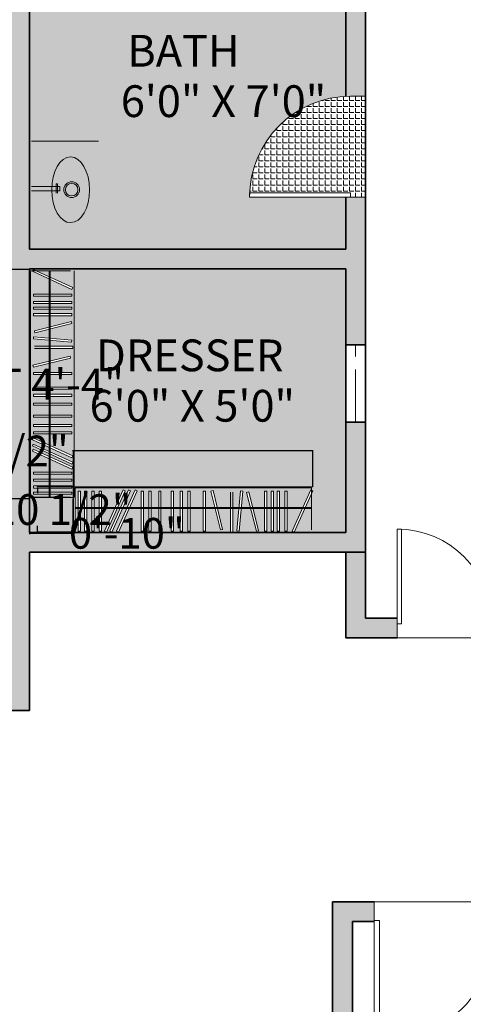
# Model space of a CAD drawing. Units: inches. Extents: x 2167 to 2589, y 1680 to 2489.
# Tile 36 of 38: x 2346 to 2447, y 2143 to 2367. Entities that reach past the tile are written whole.
import ezdxf

# ---------------------------------------------------------------- set-up
doc = ezdxf.new("R2010")
doc.units = ezdxf.units.IN
doc.header["$MEASUREMENT"] = 0
doc.linetypes.add('ACAD_ISO02W100', pattern=[15, 12, -3])
doc.layers.get('0').update_dxf_attribs({"color": 250})
for name, color, linetype, lineweight in [('A-ANNO-DIMS', 2, 'Continuous', 18), ('A-AREA-IDEN', 7, 'Continuous', 18), ('A-DOOR', 4, 'Continuous', 18), ('A-FLOR-FIXT', 8, 'Continuous', 18), ('A-FLOR-TILE-PATT', 252, 'Continuous', 13), ('A-WALL-OVHD', 8, 'ACAD_ISO02W100', 18), ('A-WALL-PATT', 250, 'Continuous', 13), ('closet', 250, 'Continuous', 18), ('walls', 7, 'Continuous', 35)]:
    doc.layers.add(name, color=color, linetype=linetype, lineweight=lineweight)
for name, color, linetype, lineweight, true_color in [('A-FLOR-FIXT-PATT', 7, 'Continuous', 13, 0xebebeb), ('A-FLOR-PATT', 254, 'Continuous', 13, 0xfeeab9), ('A-FURN-FIXD-PATT', 33, 'Continuous', 13, 0xcd8e5c)]:
    doc.layers.add(name, color=color, linetype=linetype, lineweight=lineweight, true_color=true_color)
doc.styles.get("Standard").update_dxf_attribs({"font": 'arial.ttf'})
doc.dimstyles.get("Standard").update_dxf_attribs({"dimtxt": 7, "dimasz": 0.18, "dimexe": 0.18, "dimexo": 0.0625, "dimgap": 0.09, "dimtad": 0, "dimtih": 1, "dimtoh": 1, "dimdec": 1, "dimzin": 0, "dimdsep": 46, "dimlunit": 3, "dimtxsty": 'Standard', "dimcen": 0.09, "dimadec": 0, "dimazin": 0, "dimtfac": 1, "dimtdec": 1, "dimtofl": 0, "dimtmove": 0, "dimatfit": 3, "dimfxl": 1, "dimtolj": 1, "dimtzin": 0, "dimarcsym": 0})
pattern_1 = [(0, (0, 0), (0, 1.375), [1, -0.375]), (90, (0, 0), (-1.375, 1e-16), [1, -0.375])]

# ---------------------------------------------------------------- blocks, each defined once
blk = doc.blocks.new('*U2')
for p, q in [((0, 0), (0, -6)), ((40, 0), (40, -6))]:
    blk.add_line(p, q)
blk.add_lwpolyline([(0, 0), (0, 40), (1.75, 40), (1.75, 0)], close=True)
blk.add_arc((0, 0), 40, 0, 90)
blk = doc.blocks.new('closet')
at = {"layer": 'closet'}
for p, q in [((-0.71, -5.58), (5.59, 8.19)), ((-0.23, 7.39), (-0.23, -6.57)), ((6.27, 7.88), (-0.04, -5.89)), ((5.59, 8.19), (6.27, 7.88)), ((7.92, 7.84), (8.68, 7.84)), ((7.92, 7.84), (7.92, -5.51)), ((8.68, 7.84), (8.68, -5.51)), ((10.44, 7.84), (11.2, 7.84)), ((10.44, 7.84), (10.44, -5.51)), ((11.2, 7.84), (11.2, -5.51)), ((12.45, 7.84), (13.21, 7.84)), ((12.45, 7.84), (12.45, -5.51)), ((13.21, 7.84), (13.21, -5.51)), ((14.71, 7.84), (15.47, 7.84)), ((14.71, 7.84), (14.71, -5.51)), ((15.47, 7.84), (15.47, -5.51)), ((17.44, 7.75), (18.17, 7.93)), ((17.44, 7.75), (20.73, -5.2)), ((18.17, 7.93), (21.46, -5.01)), ((23.92, 7.84), (22.75, -5.46)), ((24.67, 7.78), (23.51, -5.53)), ((23.92, 7.84), (24.67, 7.78)), ((26.09, 8.25), (26.09, -5.1)), ((26.84, 8.25), (26.84, -5.1)), ((29.49, 7.29), (32.64, -5.69)), ((30.22, 7.46), (33.37, -5.51)), ((35.23, 7.84), (35.23, -5.51)), ((35.99, 7.84), (35.99, -5.51)), ((40.33, 7.84), (40.33, -5.51)), ((41.08, 7.84), (41.08, -5.51)), ((42.85, 7.84), (42.85, -5.51)), ((43.61, 7.84), (43.61, -5.51)), ((45.9, 7.84), (45.9, -5.51)), ((46.65, 7.84), (46.65, -5.51)), ((50.07, 7.84), (50.07, -5.51)), ((50.82, 7.84), (50.82, -5.51)), ((53.32, 7.84), (53.32, -5.51)), ((54.08, 7.84), (54.08, -5.51)), ((55.9, 7.84), (55.9, -5.51)), ((56.65, 7.84), (56.65, -5.51)), ((57.99, -5.58), (64.3, 8.19)), ((64.97, 7.88), (58.67, -5.89)), ((60.19, -5.58), (66.49, 8.19)), ((67.17, 7.88), (60.87, -5.89)), ((62, -5.58), (68.3, 8.19)), ((68.98, 7.88), (62.67, -5.89)), ((69.96, 7.84), (69.96, -5.51)), ((70.72, 7.84), (70.72, -5.51)), ((72.43, 7.84), (72.43, -5.51)), ((73.19, 7.84), (73.19, -5.51)), ((74.82, 7.84), (74.82, -5.51)), ((75.57, 7.84), (75.57, -5.51)), ((76.94, 7.84), (76.94, -5.51)), ((77.69, 7.84), (77.69, -5.51)), ((56.23, 0.33), (0, 0.33)), ((56.2, 0), (0, 0)), ((56.2, 0), (78.76, 0)), ((56.23, 0.33), (78.76, 0.33)), ((-0.04, -5.89), (-0.71, -5.58)), ((21.46, -5.01), (20.73, -5.2)), ((23.51, -5.53), (22.75, -5.46)), ((33.37, -5.51), (32.64, -5.69)), ((35.99, -5.51), (35.23, -5.51)), ((41.08, -5.51), (40.33, -5.51)), ((43.61, -5.51), (42.85, -5.51)), ((46.65, -5.51), (45.9, -5.51)), ((50.82, -5.51), (50.07, -5.51)), ((54.08, -5.51), (53.32, -5.51)), ((56.65, -5.51), (55.9, -5.51)), ((58.67, -5.89), (57.99, -5.58)), ((60.87, -5.89), (60.19, -5.58)), ((62.67, -5.89), (62, -5.58)), ((70.72, -5.51), (69.96, -5.51)), ((73.19, -5.51), (72.43, -5.51)), ((75.57, -5.51), (74.82, -5.51)), ((77.69, -5.51), (76.94, -5.51))]:
    blk.add_line(p, q, dxfattribs=at)
blk = doc.blocks.new('rotated closet')
at = {"layer": 'closet'}
for p, q in [((26.32, 0.86), (27.07, 0.86)), ((29.72, -0.11), (30.45, 0.07)), ((35.46, 0.45), (36.22, 0.45)), ((40.56, 0.45), (41.31, 0.45)), ((43.08, 0.45), (43.84, 0.45)), ((46.13, 0.45), (46.88, 0.45)), ((50.3, 0.45), (51.05, 0.45)), ((53.56, 0.45), (54.31, 0.45)), ((56.13, 0.45), (56.88, 0.45)), ((64.53, 0.8), (65.2, 0.49)), ((66.72, 0.8), (67.4, 0.49)), ((68.53, 0.8), (69.21, 0.49)), ((70.19, 0.45), (70.95, 0.45)), ((72.66, 0.45), (73.42, 0.45)), ((75.05, 0.45), (75.81, 0.45)), ((77.17, 0.45), (77.92, 0.45)), ((78.99, 0), (78.99, -13.96)), ((8.91, -12.91), (8.15, -12.91)), ((11.43, -12.91), (10.67, -12.91)), ((13.44, -12.91), (12.68, -12.91)), ((15.7, -12.91), (14.94, -12.91)), ((-0.46, -14.27), (79.54, -14.27)), ((0, -13.96), (78.99, -13.96))]:
    blk.add_line(p, q, dxfattribs=at)
blk.add_blockref('closet', (0.23, -7.39), dxfattribs=at)
blk = doc.blocks.new('LAV-OVAL-WITH-TAP')
for p, q in [((6.14, 5.63), (6.14, 5.92)), ((6.14, 5.92), (8.26, 5.92)), ((8.26, 5.63), (6.14, 5.63)), ((7.69, 6.42), (6.74, 6.42)), ((6.74, 6.42), (6.74, 0)), ((7.69, 6.42), (7.69, 0))]:
    blk.add_line(p, q)
for radius in [1.79, 1.79, 1.43, 1.43, 1.43, 1.43]:
    blk.add_circle((7.46, 9.13), radius)
blk.add_ellipse((7.48, 8.9), major_axis=(7.48, 0.02), ratio=0.576535)
blk = doc.blocks.new('*D33')
at = {"layer": 'A-ANNO-DIMS', "color": 0, "lineweight": -2, "transparency": 16777216}
for p, q in [((2358.53, 2268.74), (2358.35, 2268.74)), ((2358.53, 2260.62), (2358.53, 2268.92)), ((2412.91, 2268.74), (2358.71, 2268.74)), ((2413.09, 2260.62), (2413.09, 2268.92))]:
    blk.add_line(p, q, dxfattribs=at)
at = {"layer": 'A-ANNO-DIMS', "color": 0, "transparency": 16777216}
for points in [[(2358.71, 2268.77), (2358.71, 2268.71), (2358.53, 2268.74)], [(2412.91, 2268.77), (2412.91, 2268.71), (2413.09, 2268.74)]]:
    blk.add_solid(points, dxfattribs=at)
at = {"layer": 'Defpoints', "color": 0, "transparency": 16777216}
for p in [(2358.53, 2268.74), (2358.53, 2260.56), (2413.09, 2260.56)]:
    blk.add_point(p, dxfattribs=at)
at = {"layer": 'A-ANNO-DIMS', "color": 0, "transparency": 16777216, "insert": (2319.92, 2268.74), "char_height": 7, "attachment_point": 5}
blk.add_mtext('\\A1;CLOSET 4\'-6 1/2"', dxfattribs=at)
blk = doc.blocks.new('*D34')
at = {"layer": 'A-ANNO-DIMS', "color": 0, "lineweight": -2, "transparency": 16777216}
for p, q in [((2358.47, 2260.56), (2350.17, 2260.56)), ((2350.35, 2260.38), (2350.35, 2259.11)), ((2350.35, 2250.42), (2350.35, 2251.69)), ((2358.47, 2250.24), (2350.17, 2250.24))]:
    blk.add_line(p, q, dxfattribs=at)
at = {"layer": 'A-ANNO-DIMS', "color": 0, "transparency": 16777216}
for points in [[(2350.32, 2260.38), (2350.38, 2260.38), (2350.35, 2260.56)], [(2350.32, 2250.42), (2350.38, 2250.42), (2350.35, 2250.24)]]:
    blk.add_solid(points, dxfattribs=at)
at = {"layer": 'Defpoints', "color": 0, "transparency": 16777216}
for p in [(2358.53, 2260.56), (2350.35, 2250.24), (2358.53, 2250.24)]:
    blk.add_point(p, dxfattribs=at)
at = {"layer": 'A-ANNO-DIMS', "color": 0, "transparency": 16777216, "insert": (2350.35, 2255.4), "char_height": 7, "attachment_point": 5}
blk.add_mtext('\\A1;0\'-10 1/2"', dxfattribs=at)
blk = doc.blocks.new('*D37')
at = {"layer": 'A-ANNO-DIMS', "color": 0, "lineweight": -2, "transparency": 16777216}
for p, q in [((2348.49, 2310.05), (2340.54, 2310.05)), ((2340.72, 2309.87), (2340.72, 2287.66)), ((2340.72, 2258.02), (2340.72, 2280.23)), ((2348.49, 2257.84), (2340.54, 2257.84))]:
    blk.add_line(p, q, dxfattribs=at)
at = {"layer": 'A-ANNO-DIMS', "color": 0, "transparency": 16777216}
for points in [[(2340.69, 2309.87), (2340.75, 2309.87), (2340.72, 2310.05)], [(2340.69, 2258.02), (2340.75, 2258.02), (2340.72, 2257.84)]]:
    blk.add_solid(points, dxfattribs=at)
at = {"layer": 'Defpoints', "color": 0, "transparency": 16777216}
for p in [(2348.55, 2310.05), (2340.72, 2257.84), (2348.55, 2257.84)]:
    blk.add_point(p, dxfattribs=at)
at = {"layer": 'A-ANNO-DIMS', "color": 0, "transparency": 16777216, "insert": (2340.72, 2283.95), "char_height": 7, "attachment_point": 5}
blk.add_mtext('\\A1;CLOSET 4\'-4"', dxfattribs=at)
blk = doc.blocks.new('*D38')
at = {"layer": 'A-ANNO-DIMS', "color": 0, "lineweight": -2, "transparency": 16777216}
for p, q in [((2348.55, 2257.78), (2348.55, 2249.83)), ((2358.42, 2257.78), (2358.42, 2249.83)), ((2348.73, 2250.01), (2358.24, 2250.01)), ((2358.42, 2250.01), (2358.6, 2250.01))]:
    blk.add_line(p, q, dxfattribs=at)
at = {"layer": 'A-ANNO-DIMS', "color": 0, "transparency": 16777216}
for points in [[(2348.73, 2250.04), (2348.73, 2249.98), (2348.55, 2250.01)], [(2358.24, 2250.04), (2358.24, 2249.98), (2358.42, 2250.01)]]:
    blk.add_solid(points, dxfattribs=at)
at = {"layer": 'Defpoints', "color": 0, "transparency": 16777216}
for p in [(2348.55, 2257.84), (2358.42, 2257.84), (2358.42, 2250.01)]:
    blk.add_point(p, dxfattribs=at)
at = {"layer": 'A-ANNO-DIMS', "color": 0, "transparency": 16777216, "insert": (2370.71, 2250.01), "char_height": 7, "attachment_point": 5}
blk.add_mtext('\\A1;0\'-10"', dxfattribs=at)

msp = doc.modelspace()

# ---------------------------------------------------------------- hatches: boundary and pattern name
at = {"layer": 'A-FLOR-FIXT-PATT'}
h = msp.add_hatch(color=256, dxfattribs=at)
h.dxf.hatch_style = 1
edge = h.paths.add_edge_path()
edge.add_line((2364.26, 2318.3), (2364.26, 2339.2))
edge.add_line((2364.26, 2339.2), (2349, 2339.2))
edge.add_line((2349, 2339.2), (2349, 2328.91))
edge.add_line((2349, 2328.91), (2353.6, 2328.91))
edge.add_ellipse((2357.9, 2328.17), major_axis=(0.02, -7.48), ratio=0.576535, start_angle=272.6137, end_angle=620.1108, ccw=False)
edge.add_line((2353.59, 2327.96), (2349, 2327.96))
edge.add_line((2349, 2327.96), (2349, 2318.3))
edge.add_line((2349, 2318.3), (2364.26, 2318.3))
h = msp.add_hatch(color=256, dxfattribs=at)
h.dxf.hatch_style = 1
edge = h.paths.add_edge_path()
edge.add_ellipse((2357.9, 2328.17), major_axis=(0.02, -7.48), ratio=0.576535, start_angle=272.6137, end_angle=260.1108)
edge.add_line((2353.6, 2328.91), (2354.63, 2328.91))
edge.add_line((2354.63, 2328.91), (2354.63, 2329.51))
edge.add_line((2354.63, 2329.51), (2354.92, 2329.51))
edge.add_line((2354.92, 2329.51), (2354.92, 2328.91))
edge.add_line((2354.92, 2328.91), (2355.42, 2328.91))
edge.add_line((2355.42, 2328.91), (2355.42, 2327.96))
edge.add_line((2355.42, 2327.96), (2353.59, 2327.96))
h.paths.add_polyline_path([(2358.14, 2326.4, -1), (2358.14, 2329.97, -1)], flags=16)
h.paths.add_polyline_path([(2358.14, 2329.61, -1), (2358.14, 2326.76, -1)], flags=0)
h.paths.add_polyline_path([(2358.14, 2326.76, 1), (2358.14, 2329.61, 1)], flags=0)
edge = h.paths.add_edge_path()
edge.add_line((2354.63, 2327.96), (2354.63, 2328.91))
edge.add_line((2354.63, 2328.91), (2353.6, 2328.91))
edge.add_ellipse((2357.9, 2328.17), major_axis=(0.02, -7.48), ratio=0.576535, start_angle=260.1108, end_angle=272.6137)
edge.add_line((2353.59, 2327.96), (2354.63, 2327.96))
h.paths.add_polyline_path([(2355.42, 2327.96), (2355.42, 2328.91), (2354.92, 2328.91), (2354.92, 2327.96)], flags=17)
h.paths.add_polyline_path([(2354.92, 2327.96), (2354.92, 2328.91), (2354.63, 2328.91), (2354.63, 2327.96)], flags=17)
h.paths.add_polyline_path([(2354.92, 2328.91), (2354.92, 2329.51), (2354.63, 2329.51), (2354.63, 2328.91)], flags=17)
edge = h.paths.add_edge_path()
edge.add_ellipse((2357.9, 2328.17), major_axis=(0.02, -7.48), ratio=0.576535, start_angle=260.1108, end_angle=272.6137, ccw=False)
edge.add_line((2353.6, 2328.91), (2349, 2328.91))
edge.add_line((2349, 2328.91), (2349, 2327.96))
edge.add_line((2349, 2327.96), (2353.59, 2327.96))
h = msp.add_hatch(color=256, dxfattribs=at)
h.dxf.hatch_style = 1
h.paths.add_polyline_path([(2358.14, 2329.61, 1), (2358.14, 2326.76, 1)], flags=0)
h.paths.add_polyline_path([(2358.14, 2329.97, 1), (2358.14, 2326.4, 1)])
h.paths.add_polyline_path([(2358.14, 2329.61, -1), (2358.14, 2326.76, -1)], flags=16)
h = msp.add_hatch(color=256, dxfattribs=at)
h.dxf.hatch_style = 1
h.paths.add_polyline_path([(2358.14, 2329.61, 1), (2358.14, 2326.76, 1)])
at = {"layer": 'A-FLOR-PATT'}
h = msp.add_hatch(color=256, dxfattribs=at)
h.dxf.hatch_style = 1
h.paths.add_polyline_path([(2420.55, 2310.19), (2349.46, 2310.19), (2349.4, 2310.05), (2350.08, 2309.74), (2353.25, 2309.74), (2353.25, 2308.29), (2358.7, 2305.79), (2358.7, 2260.56), (2412.76, 2260.56), (2412.76, 2259.82), (2413.09, 2259.67), (2412.76, 2258.96), (2412.76, 2255.64), (2411.24, 2255.64), (2408.75, 2250.19), (2420.55, 2250.19)])
at = {"layer": 'A-FLOR-TILE-PATT'}
h = msp.add_hatch(dxfattribs=at)
h.set_pattern_fill('ANGLE', color=256, scale=5)
h.set_pattern_definition(pattern_1)
h.paths.add_polyline_path([(2420.55, 2398.69), (2348.55, 2398.69), (2348.55, 2314.69), (2420.55, 2314.69), (2420.55, 2326.49), (2398.64, 2326.49), (2398.64, 2327.5), (2398.66, 2327.5, -0.388161), (2420.55, 2349.43)])
h.paths.add_polyline_path([(2379.26, 2371.69), (2358.26, 2371.69), (2358.26, 2373.69), (2358.76, 2373.69), (2358.76, 2383.69), (2358.26, 2383.69), (2358.26, 2385.69), (2358.76, 2385.69, -0.206081), (2365.76, 2391.29), (2365.76, 2393.69), (2364.76, 2393.69), (2364.76, 2394.69), (2362.76, 2394.69), (2362.76, 2395.69), (2374.76, 2395.69), (2374.76, 2394.69), (2372.76, 2394.69), (2372.76, 2393.69), (2371.76, 2393.69), (2371.76, 2391.29, -0.206081), (2378.76, 2385.69), (2379.26, 2385.69), (2379.26, 2383.69), (2378.76, 2383.69), (2378.76, 2373.69), (2379.26, 2373.69)], flags=16)
edge = h.paths.add_edge_path(flags=16)
edge.add_ellipse((2357.9, 2328.17), major_axis=(0.02, -7.48), ratio=0.576535, start_angle=272.6137, end_angle=620.1108, ccw=False)
edge.add_ellipse((2357.9, 2328.17), major_axis=(0.02, -7.48), ratio=0.576535, start_angle=260.1108, end_angle=272.6137, ccw=False)
h.paths.add_polyline_path([(2359.92, 2328.19, -1), (2356.35, 2328.19, -1)], flags=0)
h.paths.add_polyline_path([(2356.71, 2328.19, -1), (2359.56, 2328.19, -1)], flags=0)
h.paths.add_polyline_path([(2355.42, 2328.91), (2355.42, 2327.96), (2354.63, 2327.96), (2354.63, 2329.51), (2354.92, 2329.51), (2354.92, 2328.91)], flags=0)
h = msp.add_hatch(dxfattribs=at)
h.set_pattern_fill('ANGLE', color=256, scale=5)
h.set_pattern_definition(pattern_1)
h.paths.add_polyline_path([(2425.05, 2349.45), (2421.6, 2349.45, 0.401453), (2398.66, 2327.5), (2421.6, 2327.5), (2421.6, 2326.49), (2425.05, 2326.49)])
at = {"layer": 'A-FURN-FIXD-PATT'}
h = msp.add_hatch(color=256, dxfattribs=at)
h.dxf.hatch_style = 1
h.paths.add_polyline_path([(2349.2, 2268.7), (2349.4, 2269.14), (2353.04, 2267.47), (2353.04, 2268.12), (2349.2, 2269.88), (2349.4, 2270.32), (2353.04, 2268.65), (2353.04, 2269.55), (2349.2, 2271.31), (2349.4, 2271.75), (2353.04, 2270.08), (2353.04, 2272.63), (2349.44, 2272.63), (2349.44, 2273.12), (2353.04, 2273.12), (2353.04, 2274.3), (2349.44, 2274.3), (2349.44, 2274.8), (2353.04, 2274.8), (2353.04, 2276.43), (2349.44, 2276.43), (2349.44, 2276.92), (2353.04, 2276.92), (2353.04, 2279.15), (2349.44, 2279.15), (2349.44, 2279.64), (2353.04, 2279.64), (2353.04, 2281.14), (2349.44, 2281.14), (2349.44, 2281.63), (2353.04, 2281.63), (2353.04, 2282.78), (2349.44, 2282.78), (2349.44, 2283.28), (2353.04, 2283.28), (2353.04, 2286.11), (2349.44, 2286.11), (2349.44, 2286.6), (2353.04, 2286.6), (2353.04, 2288.69), (2349.44, 2287.81), (2349.32, 2288.29), (2353.04, 2289.2), (2353.04, 2293.93), (2349.43, 2294.25), (2349.47, 2294.74), (2353.04, 2294.43), (2353.04, 2296.42), (2349.77, 2295.58), (2349.65, 2296.06), (2353.04, 2296.93), (2353.04, 2299.5), (2349.44, 2299.5), (2349.44, 2299.99), (2353.04, 2299.99), (2353.04, 2300.97), (2349.44, 2300.97), (2349.44, 2301.47), (2353.04, 2301.47), (2353.04, 2302.28), (2349.44, 2302.28), (2349.44, 2302.77), (2353.04, 2302.77), (2353.04, 2303.93), (2349.44, 2303.93), (2349.44, 2304.42), (2353.04, 2304.42), (2353.04, 2307.85), (2349.2, 2309.61), (2349.25, 2309.74), (2348.75, 2309.74), (2348.75, 2258.2), (2353.04, 2258.2), (2353.04, 2258.9), (2349.44, 2258.9), (2349.44, 2259.39), (2353.04, 2259.39), (2353.04, 2260.28), (2349.44, 2260.28), (2349.44, 2260.77), (2353.04, 2260.77), (2353.04, 2261.84), (2349.44, 2261.84), (2349.44, 2262.33), (2353.04, 2262.33), (2353.04, 2263.45), (2349.44, 2263.45), (2349.44, 2263.94), (2353.04, 2263.94), (2353.04, 2266.94)])
h.paths.add_polyline_path([(2353.25, 2266.84), (2353.25, 2263.94), (2358.15, 2263.94), (2358.15, 2263.45), (2353.25, 2263.45), (2353.25, 2262.33), (2358.15, 2262.33), (2358.15, 2261.84), (2353.25, 2261.84), (2353.25, 2260.77), (2358.15, 2260.77), (2358.15, 2260.28), (2353.25, 2260.28), (2353.25, 2259.39), (2358.15, 2259.39), (2358.15, 2258.9), (2353.25, 2258.9), (2353.25, 2258.2), (2357.86, 2258.2), (2358.42, 2258.2), (2358.7, 2258.2), (2358.7, 2309.74), (2350.08, 2309.74), (2358.38, 2305.94), (2358.18, 2305.5), (2353.25, 2307.75), (2353.25, 2304.42), (2358.15, 2304.42), (2358.15, 2303.93), (2353.25, 2303.93), (2353.25, 2302.77), (2358.15, 2302.77), (2358.15, 2302.28), (2353.25, 2302.28), (2353.25, 2301.47), (2358.15, 2301.47), (2358.15, 2300.97), (2353.25, 2300.97), (2353.25, 2299.99), (2358.15, 2299.99), (2358.15, 2299.5), (2353.25, 2299.5), (2353.25, 2296.98), (2358.09, 2298.21), (2358.21, 2297.73), (2353.25, 2296.47), (2353.25, 2294.41), (2358.15, 2293.98), (2358.11, 2293.49), (2353.25, 2293.91), (2353.25, 2292.57), (2358.42, 2292.57), (2358.42, 2292.07), (2353.25, 2292.07), (2353.25, 2289.25), (2357.79, 2290.35), (2357.91, 2289.87), (2353.25, 2288.74), (2353.25, 2286.6), (2358.15, 2286.6), (2358.15, 2286.11), (2353.25, 2286.11), (2353.25, 2283.28), (2358.15, 2283.28), (2358.15, 2282.78), (2353.25, 2282.78), (2353.25, 2281.63), (2358.15, 2281.63), (2358.15, 2281.14), (2353.25, 2281.14), (2353.25, 2279.64), (2358.15, 2279.64), (2358.15, 2279.15), (2353.25, 2279.15), (2353.25, 2276.92), (2358.15, 2276.92), (2358.15, 2276.43), (2353.25, 2276.43), (2353.25, 2274.8), (2358.15, 2274.8), (2358.15, 2274.3), (2353.25, 2274.3), (2353.25, 2273.12), (2358.15, 2273.12), (2358.15, 2272.63), (2353.25, 2272.63), (2353.25, 2269.98), (2358.38, 2267.64), (2358.18, 2267.2), (2353.25, 2269.45), (2353.25, 2268.55), (2358.38, 2266.21), (2358.18, 2265.76), (2353.25, 2268.02), (2353.25, 2267.37), (2358.38, 2265.02), (2358.18, 2264.58)])
h = msp.add_hatch(color=256, dxfattribs=at)
h.dxf.hatch_style = 1
h.paths.add_polyline_path([(2369.87, 2259.88), (2370.33, 2259.67), (2368.59, 2255.87), (2369.27, 2255.87), (2371.11, 2259.88), (2371.57, 2259.67), (2369.83, 2255.87), (2370.77, 2255.87), (2372.6, 2259.88), (2373.06, 2259.67), (2371.32, 2255.87), (2373.98, 2255.87), (2373.98, 2259.63), (2374.49, 2259.63), (2374.49, 2255.87), (2375.73, 2255.87), (2375.73, 2259.63), (2376.25, 2259.63), (2376.25, 2255.87), (2377.95, 2255.87), (2377.95, 2259.63), (2378.47, 2259.63), (2378.47, 2255.87), (2380.8, 2255.87), (2380.8, 2259.63), (2381.31, 2259.63), (2381.31, 2255.87), (2382.87, 2255.87), (2382.87, 2259.63), (2383.39, 2259.63), (2383.39, 2255.87), (2384.59, 2255.87), (2384.59, 2259.63), (2385.11, 2259.63), (2385.11, 2255.87), (2388.07, 2255.87), (2388.07, 2259.63), (2388.58, 2259.63), (2388.58, 2255.87), (2390.76, 2255.87), (2389.85, 2259.63), (2390.35, 2259.75), (2391.29, 2255.87), (2396.25, 2255.87), (2396.57, 2259.64), (2397.09, 2259.59), (2396.76, 2255.87), (2398.84, 2255.87), (2397.97, 2259.28), (2398.47, 2259.41), (2399.37, 2255.87), (2402.06, 2255.87), (2402.06, 2259.63), (2402.57, 2259.63), (2402.57, 2255.87), (2403.6, 2255.87), (2403.6, 2259.63), (2404.11, 2259.63), (2404.11, 2255.87), (2404.97, 2255.87), (2404.97, 2259.63), (2405.48, 2259.63), (2405.48, 2255.87), (2406.69, 2255.87), (2406.69, 2259.63), (2407.2, 2259.63), (2407.2, 2255.87), (2410.79, 2255.87), (2412.63, 2259.88), (2412.76, 2259.82), (2412.76, 2260.35), (2358.91, 2260.35), (2358.91, 2255.87), (2359.63, 2255.87), (2359.63, 2259.63), (2360.15, 2259.63), (2360.15, 2255.87), (2361.08, 2255.87), (2361.08, 2259.63), (2361.6, 2259.63), (2361.6, 2255.87), (2362.71, 2255.87), (2362.71, 2259.63), (2363.22, 2259.63), (2363.22, 2255.87), (2364.39, 2255.87), (2364.39, 2259.63), (2364.9, 2259.63), (2364.9, 2255.87), (2368.04, 2255.87)])
h.paths.add_polyline_path([(2367.93, 2255.64), (2364.9, 2255.64), (2364.9, 2250.52), (2364.39, 2250.52), (2364.39, 2255.64), (2363.22, 2255.64), (2363.22, 2250.52), (2362.71, 2250.52), (2362.71, 2255.64), (2361.6, 2255.64), (2361.6, 2250.52), (2361.08, 2250.52), (2361.08, 2255.64), (2360.15, 2255.64), (2360.15, 2250.52), (2359.63, 2250.52), (2359.63, 2255.64), (2358.91, 2255.64), (2358.91, 2250.83), (2358.91, 2250.25), (2358.91, 2249.95), (2412.76, 2249.95), (2412.76, 2258.96), (2408.79, 2250.28), (2408.33, 2250.5), (2410.68, 2255.64), (2407.2, 2255.64), (2407.2, 2250.52), (2406.69, 2250.52), (2406.69, 2255.64), (2405.48, 2255.64), (2405.48, 2250.52), (2404.97, 2250.52), (2404.97, 2255.64), (2404.11, 2255.64), (2404.11, 2250.52), (2403.6, 2250.52), (2403.6, 2255.64), (2402.57, 2255.64), (2402.57, 2250.52), (2402.06, 2250.52), (2402.06, 2255.64), (2399.43, 2255.64), (2400.71, 2250.59), (2400.21, 2250.46), (2398.9, 2255.64), (2396.74, 2255.64), (2396.3, 2250.52), (2395.78, 2250.57), (2396.23, 2255.64), (2394.82, 2255.64), (2394.82, 2250.24), (2394.3, 2250.24), (2394.3, 2255.64), (2391.35, 2255.64), (2392.5, 2250.9), (2392, 2250.78), (2390.82, 2255.64), (2388.58, 2255.64), (2388.58, 2250.52), (2388.07, 2250.52), (2388.07, 2255.64), (2385.11, 2255.64), (2385.11, 2250.52), (2384.59, 2250.52), (2384.59, 2255.64), (2383.39, 2255.64), (2383.39, 2250.52), (2382.87, 2250.52), (2382.87, 2255.64), (2381.31, 2255.64), (2381.31, 2250.52), (2380.8, 2250.52), (2380.8, 2255.64), (2378.47, 2255.64), (2378.47, 2250.52), (2377.95, 2250.52), (2377.95, 2255.64), (2376.25, 2255.64), (2376.25, 2250.52), (2375.73, 2250.52), (2375.73, 2255.64), (2374.49, 2255.64), (2374.49, 2250.52), (2373.98, 2250.52), (2373.98, 2255.64), (2371.22, 2255.64), (2368.77, 2250.28), (2368.31, 2250.5), (2370.66, 2255.64), (2369.72, 2255.64), (2367.27, 2250.28), (2366.81, 2250.5), (2369.17, 2255.64), (2368.49, 2255.64), (2366.04, 2250.28), (2365.58, 2250.5)])
h = msp.add_hatch(color=256, dxfattribs=at)
h.dxf.hatch_style = 1
h.paths.add_polyline_path([(2358.48, 2258.16), (2348.55, 2258.16), (2348.55, 2257.84), (2348.55, 2250.19), (2358.48, 2250.19)])
at = {"layer": 'A-WALL-PATT'}
h = msp.add_hatch(color=256, dxfattribs=at)
h.dxf.hatch_style = 1
h.paths.add_polyline_path([(2471.54, 2407.69), (2405.59, 2407.69), (2405.59, 2398.69), (2420.55, 2398.69), (2420.55, 2349.43, -0.011499), (2421.6, 2349.45), (2425.05, 2349.45), (2425.05, 2398.69), (2471.54, 2398.69)])
h.paths.add_polyline_path([(2420.55, 2250.19), (2348.55, 2250.19), (2348.55, 2310.19), (2420.55, 2310.19)], flags=16)
h.paths.add_polyline_path([(2320.06, 2212.92, -0.014764), (2320.1, 2214.19), (2224.05, 2214.19), (2224.05, 2346.19), (2250.86, 2346.19), (2250.86, 2350.69), (2224.05, 2350.69), (2224.05, 2398.69), (2250.76, 2398.69), (2250.76, 2407.69), (2215.05, 2407.69), (2215.05, 2179.66), (2218.49, 2179.66), (2224.05, 2179.66), (2224.05, 2209.69), (2314.05, 2209.69), (2314.05, 2202.4), (2314.78, 2202.4), (2318.55, 2202.4), (2318.55, 2209.69), (2320.06, 2209.69)])
h.paths.add_polyline_path([(2310.92, 2349.42, -0.014764), (2310.96, 2350.69), (2297.23, 2350.69), (2297.23, 2346.19), (2310.92, 2346.19)], flags=17)
h.paths.add_polyline_path([(2425.05, 2275.27), (2420.55, 2275.27), (2420.55, 2292.87), (2425.05, 2292.87), (2425.05, 2326.49), (2421.6, 2326.49), (2420.55, 2326.49), (2420.55, 2314.69), (2348.55, 2314.69), (2348.55, 2398.69), (2373.55, 2398.69), (2373.55, 2404.36), (2373.55, 2407.69), (2297.68, 2407.69), (2297.68, 2398.69), (2344.05, 2398.69), (2344.05, 2350.69), (2332.45, 2350.69), (2332.45, 2349.42), (2332.45, 2346.19), (2344.05, 2346.19), (2344.05, 2214.19), (2341.59, 2214.19), (2341.59, 2212.92), (2341.59, 2209.69), (2348.55, 2209.69), (2348.55, 2245.69), (2425.05, 2245.69)])
h = msp.add_hatch(color=256, dxfattribs=at)
h.dxf.hatch_style = 1
h.paths.add_polyline_path([(2575.05, 2029.69), (2422.05, 2029.69), (2422.05, 2161.69), (2427.02, 2161.69), (2427.02, 2161.94), (2427.02, 2166.19), (2417.55, 2166.19), (2417.55, 2025.19), (2575.05, 2025.19)])
h.paths.add_polyline_path([(2575.05, 2166.19), (2503.01, 2166.19), (2503.01, 2161.69), (2575.05, 2161.69)], flags=17)
h.paths.add_polyline_path([(2575.05, 2161.69), (2566.05, 2161.69), (2566.05, 2029.69), (2575.05, 2029.69)], flags=17)
h.paths.add_polyline_path([(2575.05, 2025.19), (2566.05, 2025.19), (2566.05, 1869.19), (2575.05, 1869.19)])
h.paths.add_polyline_path([(2575.05, 1869.19), (2566.05, 1869.19), (2447.7, 1869.19, -0.014764), (2447.74, 1867.92), (2447.74, 1864.69), (2575.05, 1864.69)])
h.paths.add_polyline_path([(2530.05, 1864.69), (2525.55, 1864.69), (2525.55, 1816.69), (2452.05, 1816.69), (2452.05, 1812.19), (2530.05, 1812.19)])
h.paths.add_polyline_path([(2455.04, 1830.65), (2452.05, 1830.65), (2452.05, 1816.69), (2455.04, 1816.69)], flags=17)
h.paths.add_polyline_path([(2575.05, 1864.69), (2566.05, 1864.69), (2566.05, 1788.19), (2456.1, 1788.19), (2456.1, 1783.94, -0.042065), (2455.7, 1779.19), (2527.68, 1779.19), (2527.68, 1687.69), (2532.18, 1687.69), (2532.18, 1779.19), (2575.05, 1779.19)])
h.paths.add_polyline_path([(2421.87, 1696.69), (2416.11, 1696.69), (2416.11, 1687.69), (2421.87, 1687.69)])
h.paths.add_polyline_path([(2375.61, 1696.69), (2369.84, 1696.69), (2369.84, 1687.69), (2375.61, 1687.69)])
h.paths.add_polyline_path([(2425.05, 2245.69), (2420.55, 2245.69), (2420.55, 2226.19), (2432.29, 2226.19), (2432.29, 2229.42), (2432.29, 2230.69), (2425.05, 2230.69)])
h.paths.add_polyline_path([(2224.05, 2151.19), (2318.55, 2151.19), (2318.55, 2177.3), (2314.78, 2177.3, -0.007324), (2314.05, 2177.32), (2314.05, 2155.69), (2224.05, 2155.69), (2224.05, 2157.46), (2215.05, 2157.46), (2215.05, 2103.59), (2218.97, 2103.59), (2224.05, 2103.59)])

# ---------------------------------------------------------------- linework, layer by layer
at = {"layer": 'A-DOOR'}
for p, q in [((2432.29, 2226.19), (2453.82, 2226.19)), ((2427.02, 2166.19), (2455.38, 2166.19))]:
    msp.add_line(p, q, dxfattribs=at)
at = {"layer": 'A-FLOR-FIXT'}
msp.add_line((2364.26, 2339.2), (2349, 2339.2), dxfattribs=at)
at = {"layer": 'A-WALL-OVHD'}
msp.add_line((2422.8, 2275.27), (2422.8, 2292.87), dxfattribs=at)
at = {"layer": 'closet'}
for p, q in [((2348.55, 2257.84), (2348.55, 2310.04)), ((2348.75, 2309.74), (2348.75, 2258.2)), ((2348.75, 2309.74), (2357.86, 2309.74)), ((2358.7, 2309.74), (2358.7, 2258.16)), ((2358.48, 2260.77), (2358.15, 2260.77)), ((2358.48, 2250.19), (2358.48, 2260.77)), ((2358.53, 2260.56), (2413.07, 2260.56)), ((2358.53, 2260.56), (2358.53, 2250.19)), ((2358.7, 2258.16), (2358.7, 2260.56)), ((2412.76, 2260.35), (2358.91, 2260.35)), ((2412.76, 2260.35), (2412.76, 2250.83)), ((2358.47, 2258.16), (2348.55, 2258.16)), ((2348.55, 2258.16), (2348.55, 2257.84)), ((2348.75, 2258.2), (2357.86, 2258.2))]:
    msp.add_line(p, q, dxfattribs=at)
at = {"layer": 'walls'}
for p, q in [((2348.55, 2314.69), (2348.55, 2398.69)), ((2420.55, 2349.43), (2420.55, 2398.69)), ((2425.05, 2230.69), (2425.05, 2398.69)), ((2420.55, 2314.69), (2420.55, 2326.49)), ((2348.55, 2314.69), (2420.55, 2314.69)), ((2348.55, 2310.19), (2420.55, 2310.19)), ((2348.55, 2250.19), (2348.55, 2310.19)), ((2420.55, 2250.19), (2420.55, 2310.19)), ((2420.55, 2292.87), (2425.05, 2292.87)), ((2420.55, 2275.27), (2425.05, 2275.27)), ((2348.55, 2250.19), (2420.55, 2250.19)), ((2348.55, 2209.69), (2348.55, 2245.69)), ((2348.55, 2245.69), (2425.05, 2245.69)), ((2420.55, 2226.19), (2420.55, 2245.69)), ((2425.05, 2230.69), (2432.29, 2230.69)), ((2420.55, 2226.19), (2432.29, 2226.19)), ((2318.55, 2209.69), (2348.55, 2209.69)), ((2417.55, 2166.19), (2427.02, 2166.19)), ((2417.55, 2166.19), (2417.55, 2025.19)), ((2422.05, 2161.69), (2427.02, 2161.69)), ((2422.05, 2161.69), (2422.05, 2029.69))]:
    msp.add_line(p, q, dxfattribs=at)

# ---------------------------------------------------------------- block references
at = {"layer": 'A-DOOR'}
for p, xscale, yscale, zscale, rotation in [((2421.6, 2326.49), 0.5740396890227921, 0.5740396890227921, 0.5740396890227921, 90), ((2427.02, 2161.94), -0.7089553820317277, 0.7089553820317277, 0.7089553820317277, 180)]:
    msp.add_blockref('*U2', p, dxfattribs=dict(at, xscale=xscale, yscale=yscale, zscale=zscale, rotation=rotation))
at = {"layer": 'A-DOOR', "xscale": 0.5382298898187942, "yscale": 0.5382298898187942, "zscale": 0.5382298898187942}
msp.add_blockref('*U2', (2432.29, 2229.42), dxfattribs=at)
at = {"layer": 'A-FLOR-FIXT', "rotation": 269.9999999999934}
msp.add_blockref('LAV-OVAL-WITH-TAP', (2349, 2335.65), dxfattribs=at)
at = {"layer": 'closet'}
for p, xscale, yscale, zscale, rotation in [((2357.86, 2309.74), 0.6524297493915985, 0.6524297493915985, 0.6524297493915985, 269.9999999992008), ((2412.76, 2250.83), 0.681746927348746, 0.681746927348746, 0.681746927348746, 179.9999999992007)]:
    msp.add_blockref('rotated closet', p, dxfattribs=dict(at, xscale=xscale, yscale=yscale, zscale=zscale, rotation=rotation))

# ---------------------------------------------------------------- texts
at = {"layer": 'A-AREA-IDEN'}
for s, height, p in [('BATH', 7.227, (2370.81, 2356.19)), ('6\'0" X 7\'0"', 7.2272, (2369.33, 2344.72)), ('DRESSER', 7.227, (2363.69, 2286.88)), ('6\'0" X 5\'0"', 7.2272, (2362.22, 2275.41))]:
    msp.add_text(s, height=height, dxfattribs=at).set_placement(p)

# ---------------------------------------------------------------- dimensions: what is measured, and where the dimension line sits
at = {"layer": 'A-ANNO-DIMS'}
for base, p1, p2, angle, picture, middle in [((2340.72, 2257.84), (2348.55, 2310.05), (2348.55, 2257.84), 270, '*D37', (2340.72, 2283.95)), ((2358.53, 2268.74), (2413.09, 2260.56), (2358.53, 2260.56), 180, '*D33', (2319.92, 2268.74))]:
    dim = msp.add_linear_dim(base=base, p1=p1, p2=p2, angle=angle, text='CLOSET <>', dimstyle='Standard', override={"dimdec": 1, "dimlfac": 1, "dimrnd": 0, "dimzin": 1, "dimdsep": 46, "dimlunit": 4, "dimfrac": 2}, dxfattribs=at)
    dim.commit()
    dim.dimension.update_dxf_attribs({"geometry": picture, "text_midpoint": middle})
dim = msp.add_linear_dim(base=(2350.35, 2250.24), p1=(2358.53, 2260.56), p2=(2358.53, 2250.24), angle=270, dimstyle='Standard', override={"dimdec": 1, "dimlfac": 1, "dimrnd": 0, "dimzin": 1, "dimdsep": 46, "dimlunit": 4, "dimfrac": 2}, dxfattribs=at)
dim.commit()
dim.dimension.update_dxf_attribs({"geometry": '*D34', "text_midpoint": (2350.35, 2255.4)})
dim = msp.add_linear_dim(base=(2358.42, 2250.01), p1=(2348.55, 2257.84), p2=(2358.42, 2257.84), dimstyle='Standard', override={"dimdec": 1, "dimlfac": 1, "dimrnd": 0, "dimzin": 1, "dimdsep": 46, "dimlunit": 4, "dimfrac": 2}, dxfattribs=at)
dim.commit()
dim.dimension.update_dxf_attribs({"geometry": '*D38', "text_midpoint": (2370.71, 2250.01)})

doc.saveas('drawing.dxf')
